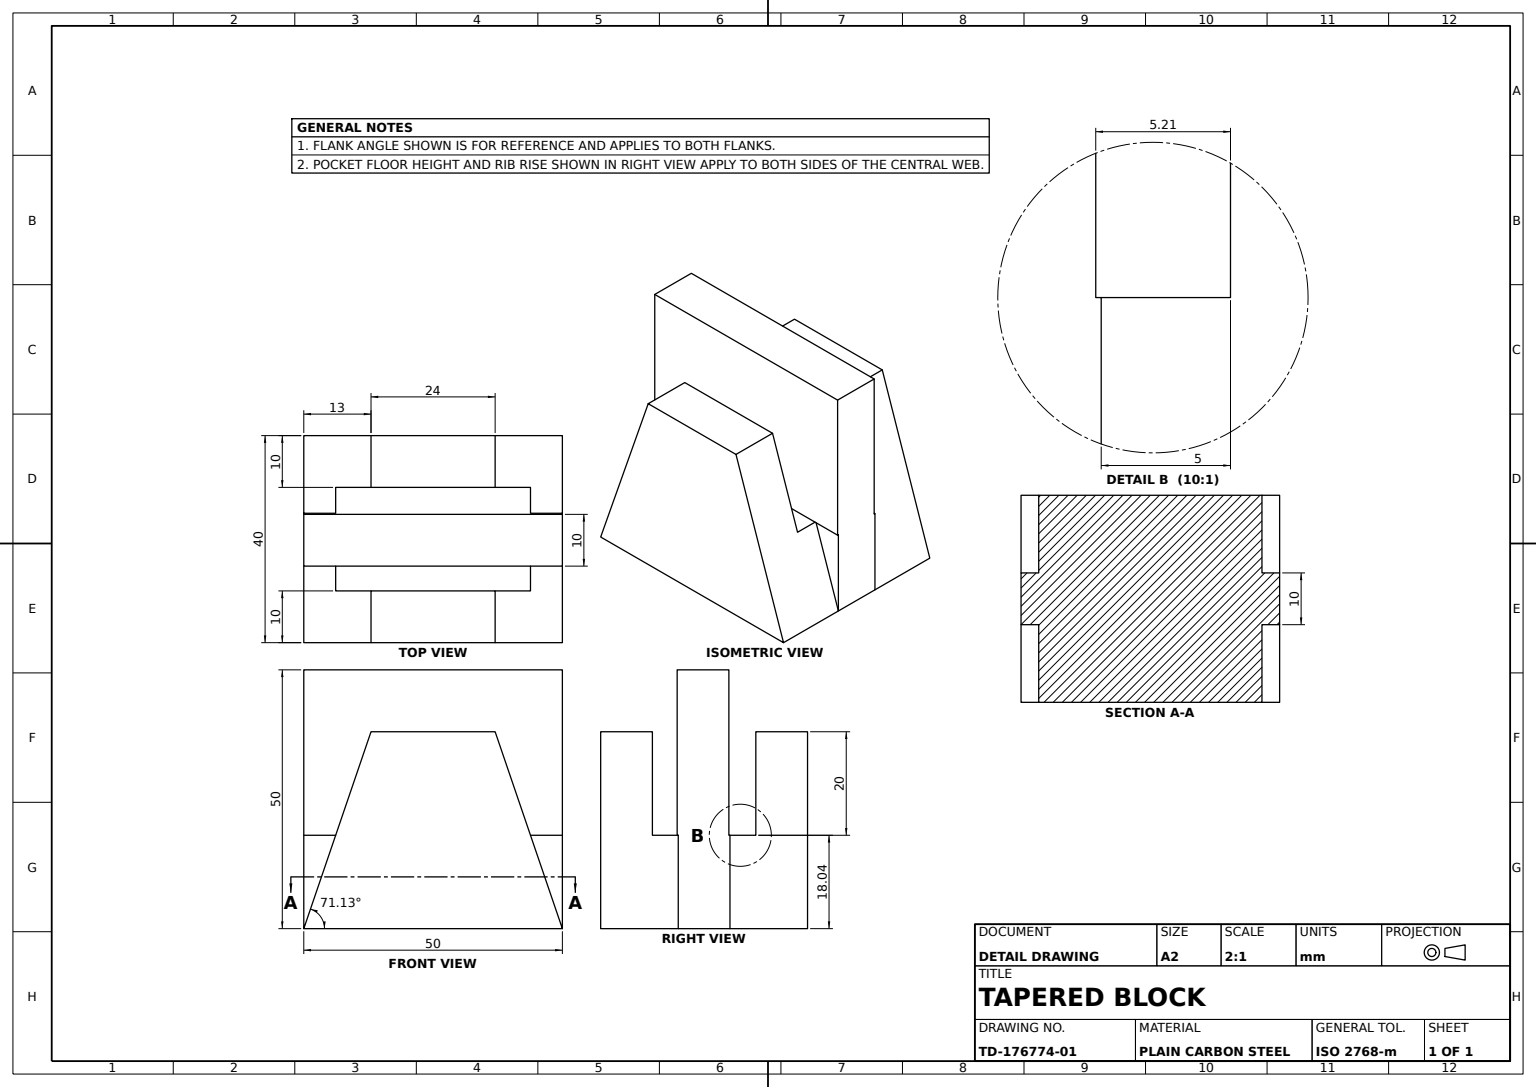
from build123d import *

# Parameters (mm, degrees)
BASE_BLOCK_40MM_DEPTH       = 40
STEP_PROFILE_CUT_SKETCH_W   = 10
STEP_PROFILE_CUT_SKETCH_H   = 11.958807021
STEP_PROFILE_CUT_DEPTH      = 69.738635424
POCKET_24MM_X_10_DEEP_DEPTH = 10
POCKET_12MM_X_10_DEEP_DEPTH = 10
TRIANGULAR_CUT_A_5MM_DEPTH  = 5
TRIANGULAR_CUT_B_5MM_DEPTH  = 5
TRIANGULAR_CUT_C_5MM_DEPTH  = 5
TRIANGULAR_CUT_D_5MM_DEPTH  = 5


with BuildPart() as part:
    # Base Profile Sketch → Base Block 40mm (new body)
    with BuildSketch(Plane.XY):
        Polygon((12, 25), (-12, 25), (-25, 25), (-25, -25), (-12, 13), (12, 13), (25, -25), (25, 25), align=None)
        Polygon((12, 13), (25, -25), (-25, -25), (-12, 13), align=None)
    extrude(amount=BASE_BLOCK_40MM_DEPTH)

    # Step Profile Cut Sketch → Step Profile Cut (cut, through all)
    with BuildSketch(Plane(origin=(25, 0, 0), x_dir=(0, 0, -1), z_dir=(1, 0, 0))):
        Polygon((-25.21106926, -6.958807021), (-25.21106926, 25), (-30, 25), (-40, 25), (-40, 13.041192979), (-30, 13.041192979), (-30, -6.958807021), align=None)
        Polygon((-10, -6.958807021), (-10, 13.041192979), (-10, 25), (-15.21106926, 25), (-15.21106926, -6.958807021), align=None)
        with Locations((-5, 19.02059649)):
            Rectangle(STEP_PROFILE_CUT_SKETCH_W, STEP_PROFILE_CUT_SKETCH_H)
    extrude(amount=-STEP_PROFILE_CUT_DEPTH, mode=Mode.SUBTRACT)

    # Pocket 24mm Sketch → Pocket 24mm x 10 Deep (cut)
    with BuildSketch(Plane(origin=(0, 0, 0), x_dir=(-1, 0, 0), z_dir=(0, 0, -1))):
        Polygon((-12, 13.041192979), (12, 13.041192979), (25, -25), (25, 25), (-25, 25), (-25, -25), align=None)
    extrude(amount=-POCKET_24MM_X_10_DEEP_DEPTH, mode=Mode.SUBTRACT)

    # Pocket 12mm Sketch → Pocket 12mm x 10 Deep (cut)
    with BuildSketch(Plane.XY.offset(40)):
        Polygon((-25, -25), (-12, 13.041192979), (12, 13.041192979), (25, -25), (25, 25), (-25, 25), align=None)
    extrude(amount=-POCKET_12MM_X_10_DEEP_DEPTH, mode=Mode.SUBTRACT)

    # Triangular Cut A Sketch → Triangular Cut A 5mm (cut)
    with BuildSketch(Plane.XY.offset(30)):
        Polygon((-25, -25), (-25, -6.958807021), (-18.834696276, -6.958807021), align=None)
    extrude(amount=-TRIANGULAR_CUT_A_5MM_DEPTH, mode=Mode.SUBTRACT)

    # Triangular Cut B Sketch → Triangular Cut B 5mm (cut)
    with BuildSketch(Plane(origin=(0, 0, 10), x_dir=(-1, 0, 0), z_dir=(0, 0, -1))):
        Polygon((25, -25), (25, -6.958807021), (18.834696276, -6.958807021), align=None)
    extrude(amount=-TRIANGULAR_CUT_B_5MM_DEPTH, mode=Mode.SUBTRACT)

    # Triangular Cut C Sketch → Triangular Cut C 5mm (cut)
    with BuildSketch(Plane(origin=(0, 0, 10), x_dir=(-1, 0, 0), z_dir=(0, 0, -1))):
        Polygon((-25, -25), (-18.834696276, -6.958807021), (-25, -6.958807021), align=None)
    extrude(amount=-TRIANGULAR_CUT_C_5MM_DEPTH, mode=Mode.SUBTRACT)

    # Triangular Cut D Sketch → Triangular Cut D 5mm (cut)
    with BuildSketch(Plane.XY.offset(30)):
        Polygon((25, -25), (25, -6.958807021), (18.834696276, -6.958807021), align=None)
    extrude(amount=-TRIANGULAR_CUT_D_5MM_DEPTH, mode=Mode.SUBTRACT)


solid = part.part
